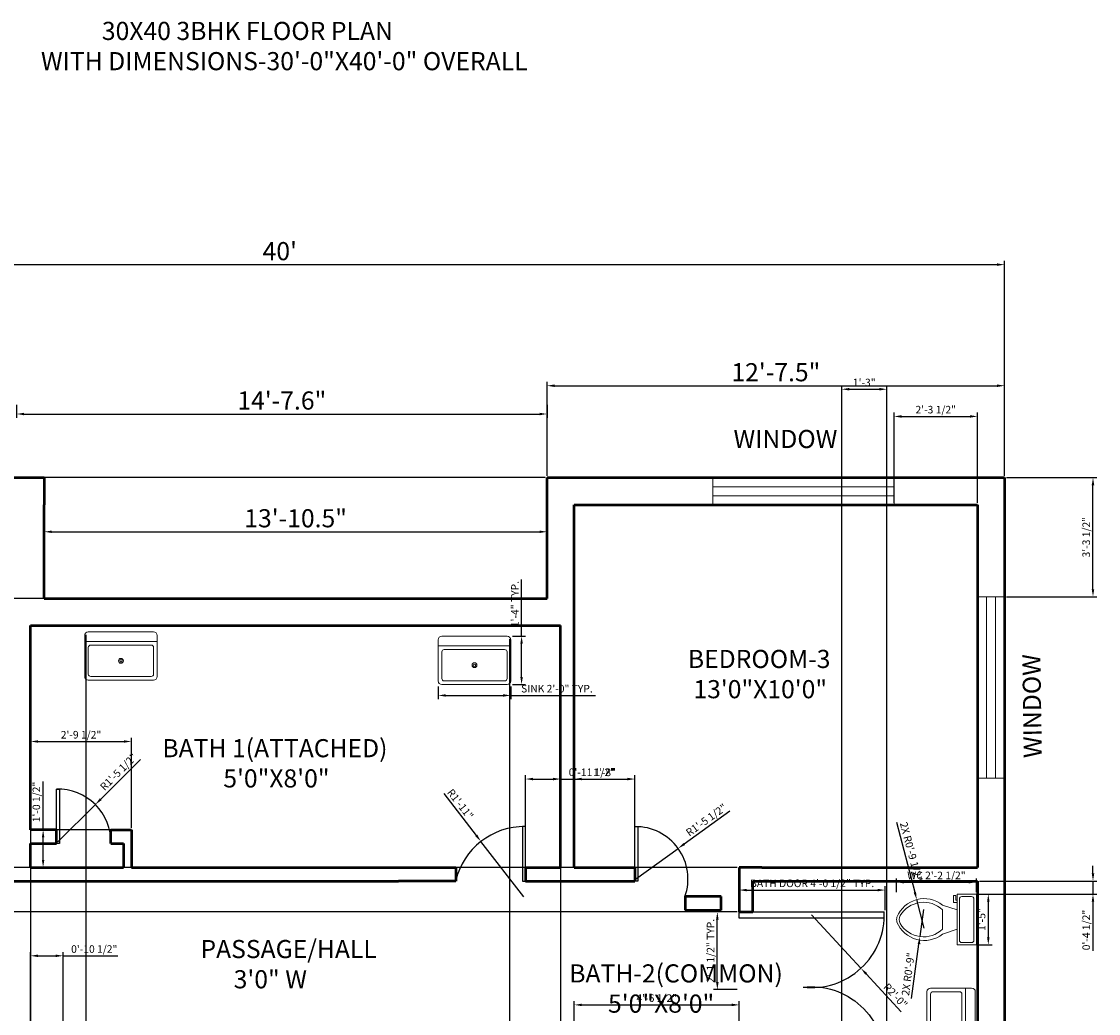
# Model space of a CAD drawing. Units: inches. Extents: x 259417 to 260009, y 246275 to 246915.
# Tile 4 of 4: x 259652 to 260009, y 246587 to 246915. Entities that reach past the tile are written whole.
import ezdxf

# ---------------------------------------------------------------- set-up
doc = ezdxf.new("R2010")
doc.units = ezdxf.units.IN
for name, color, linetype, lineweight in [('A-ANNO-DIMS', 2, 'Continuous', 18), ('A-ANNO-TEXT', 7, 'Continuous', 18), ('A-ANNO-TTLB', 7, 'Continuous', 35), ('A-AREA-IDEN', 7, 'Continuous', 25), ('A-DOOR', 3, 'Continuous', 25), ('A-FLOR-FIXT', 8, 'Continuous', 18), ('A-GLAZ', 4, 'Continuous', 18), ('A-WALL', 7, 'Continuous', 50)]:
    doc.layers.add(name, color=color, linetype=linetype, lineweight=lineweight)
doc.styles.get("Standard").update_dxf_attribs({"font": 'arial.ttf'})
doc.dimstyles.new('ISO-25', dxfattribs={"dimtxt": 2.5, "dimasz": 2.5, "dimexe": 1.25, "dimexo": 0.625, "dimtad": 1, "dimdec": 1, "dimlunit": 3, "dimtxsty": 'Standard', "dimcen": 2.5, "dimadec": 0, "dimazin": 0, "dimtfac": 1, "dimtdec": 1, "dimtmove": 0, "dimatfit": 3, "dimfxl": 1, "dimarcsym": 0})

# ---------------------------------------------------------------- blocks, each defined once
blk = doc.blocks.new('*D8')
at = {"layer": 'A-ANNO-DIMS', "color": 0, "lineweight": -2, "transparency": 16777216}
for p, q in [((259497.59, 246764.47), (259497.59, 246835.57)), ((259500.09, 246834.32), (259975.09, 246834.32)), ((259977.59, 246764.47), (259977.59, 246835.57))]:
    blk.add_line(p, q, dxfattribs=at)
at = {"layer": 'A-ANNO-DIMS', "color": 0, "transparency": 16777216}
for points in [[(259500.09, 246834.74), (259500.09, 246833.91), (259497.59, 246834.32)], [(259975.09, 246834.74), (259975.09, 246833.91), (259977.59, 246834.32)]]:
    blk.add_solid(points, dxfattribs=at)
at = {"layer": 'Defpoints', "color": 0, "transparency": 16777216}
for p in [(259977.59, 246834.32), (259497.59, 246763.84), (259977.59, 246763.84)]:
    blk.add_point(p, dxfattribs=at)
at = {"layer": 'A-ANNO-DIMS', "color": 0, "transparency": 16777216, "insert": (259737.59, 246838.01), "char_height": 6, "attachment_point": 5}
blk.add_mtext("40'", dxfattribs=at)
blk = doc.blocks.new('*D12')
at = {"layer": 'A-ANNO-DIMS', "color": 0, "lineweight": -2, "transparency": 16777216}
for p, q in [((259659.59, 246724.51), (259659.59, 246747.17)), ((259826.09, 246724.51), (259826.09, 246747.17)), ((259662.09, 246745.92), (259823.59, 246745.92))]:
    blk.add_line(p, q, dxfattribs=at)
at = {"layer": 'A-ANNO-DIMS', "color": 0, "transparency": 16777216}
for points in [[(259662.09, 246746.33), (259662.09, 246745.5), (259659.59, 246745.92)], [(259823.59, 246746.33), (259823.59, 246745.5), (259826.09, 246745.92)]]:
    blk.add_solid(points, dxfattribs=at)
at = {"layer": 'Defpoints', "color": 0, "transparency": 16777216}
for p in [(259826.09, 246745.92), (259659.59, 246723.89), (259826.09, 246723.89)]:
    blk.add_point(p, dxfattribs=at)
at = {"layer": 'A-ANNO-DIMS', "color": 0, "transparency": 16777216, "insert": (259742.84, 246749.61), "char_height": 6, "attachment_point": 5}
blk.add_mtext('13\'-10.5"', dxfattribs=at)
blk = doc.blocks.new('*D13')
at = {"layer": 'A-ANNO-DIMS', "color": 0, "lineweight": -2, "transparency": 16777216}
for p, q in [((259826.09, 246764.47), (259826.09, 246795.5)), ((259828.59, 246794.25), (259975.09, 246794.25)), ((259977.59, 246764.47), (259977.59, 246795.5))]:
    blk.add_line(p, q, dxfattribs=at)
at = {"layer": 'A-ANNO-DIMS', "color": 0, "transparency": 16777216}
for points in [[(259828.59, 246794.67), (259828.59, 246793.84), (259826.09, 246794.25)], [(259975.09, 246794.67), (259975.09, 246793.84), (259977.59, 246794.25)]]:
    blk.add_solid(points, dxfattribs=at)
at = {"layer": 'Defpoints', "color": 0, "transparency": 16777216}
for p in [(259977.59, 246794.25), (259826.09, 246763.84), (259977.59, 246763.84)]:
    blk.add_point(p, dxfattribs=at)
at = {"layer": 'A-ANNO-DIMS', "color": 0, "transparency": 16777216, "insert": (259901.84, 246797.94), "char_height": 6, "attachment_point": 5}
blk.add_mtext('12\'-7.5"', dxfattribs=at)
blk = doc.blocks.new('*D14')
at = {"layer": 'A-ANNO-DIMS', "color": 0, "lineweight": -2, "transparency": 16777216}
for p, q in [((259650.46, 246787.95), (259650.46, 246783.64)), ((259826.09, 246787.95), (259826.09, 246783.64)), ((259652.96, 246784.89), (259823.59, 246784.89))]:
    blk.add_line(p, q, dxfattribs=at)
at = {"layer": 'A-ANNO-DIMS', "color": 0, "transparency": 16777216}
for points in [[(259652.96, 246785.31), (259652.96, 246784.47), (259650.46, 246784.89)], [(259823.59, 246785.31), (259823.59, 246784.47), (259826.09, 246784.89)]]:
    blk.add_solid(points, dxfattribs=at)
at = {"layer": 'Defpoints', "color": 0, "transparency": 16777216}
for p in [(259650.46, 246788.57), (259826.09, 246788.57), (259826.09, 246784.89)]:
    blk.add_point(p, dxfattribs=at)
at = {"layer": 'A-ANNO-DIMS', "color": 0, "transparency": 16777216, "insert": (259738.27, 246788.58), "char_height": 6, "attachment_point": 5}
blk.add_mtext('14\'-7.6"', dxfattribs=at)
blk = doc.blocks.new('Toilet - top')
for p, q in [((9.5, -6), (9.5, -2)), ((-10, -8.5), (-8, -8.5)), ((-10, -9.5), (-10, -8.5)), ((-8, -8.5), (-8, -8)), ((-7, -8), (-7, -9.5)), ((-4, -8), (-6, -14)), ((4, -8), (6, -14)), ((-7, -9.5), (-10, -9.5)), ((4, -14), (-4, -14))]:
    blk.add_line(p, q)
blk.add_lwpolyline([(10.5, -8), (10.5, 0), (-10.5, 0), (-10.5, -8)], close=True)
for points in [[(-9.5, -2), (-9.5, -6)], [(8.5, -1), (-8.5, -1)], [(-8.5, -7), (8.5, -7)]]:
    blk.add_lwpolyline(points)
for centre, radius, start, end in [((-8.62, -1.88), 0.884, 81.8699, 188.1301), ((8.62, -1.88), 0.884, 351.8699, 98.1301), ((-8.62, -6.12), 0.884, 171.8699, 278.1301), ((8.62, -6.12), 0.884, 261.8699, 8.1301), ((3.52, -21.58), 12.17, 141.4691, 247.9714), ((4.2, -21.82), 11.33, 136.3677, 238.9468), ((-3.52, -21.58), 12.17, 292.0284, 38.5307), ((-4.2, -21.82), 11.33, 301.053, 43.6321), ((0, -27.88), 4, 245.7318, 294.2682), ((0, -29), 4, 254.8605, 285.1395)]:
    blk.add_arc(centre, radius, start, end)
blk = doc.blocks.new('Sink-single - 30 in top')
blk.add_line((-15, -3.999996), (15, -3.999996))
for points in [[(-13.5, 0), (13.5, 0)], [(-15, -18.499996), (-15, -1.5)], [(15, -1.5), (15, -18.499996)], [(-13.5, -17.499996), (-13.5, -6.499996)], [(-12.5, -5.499996), (12.5, -5.499996)], [(13.5, -6.499996), (13.5, -17.499996)], [(13.5, -19.999996), (-13.5, -19.999996)], [(12.5, -18.499996), (-12.5, -18.499996)]]:
    blk.add_lwpolyline(points)
for radius in [1, 0.5]:
    blk.add_circle((0, -11.999996), radius)
for centre, radius, start, end in [((-13.5, -1.5), 1.5, 90, 180), ((13.5, -1.5), 1.5, 0, 90), ((-12.5, -6.499996), 1, 90, 180), ((12.5, -6.499996), 1, 0, 90), ((-12.5, -17.499996), 1, 180, 270), ((12.5, -17.499996), 1, 270, 0), ((-13.5, -18.499996), 1.5, 180, 270), ((13.5, -18.499996), 1.5, 270, 0)]:
    blk.add_arc(centre, radius, start, end)
blk = doc.blocks.new('WIN-60x9')
for p, q in [((0, 9), (0, 0)), ((60, 9), (60, 0)), ((60, 6), (0, 6)), ((60, 3), (0, 3))]:
    blk.add_line(p, q)
blk = doc.blocks.new('DOOR-BATH-PAIRED-LEAF')
for p, q in [((0, 0), (48, 0)), ((0, -2), (0, 0)), ((48, -2), (0, -2)), ((48, -2), (48, 0))]:
    blk.add_line(p, q)
blk.add_arc((23.97, -1), 24.05, 263.254, 2.3829)
blk = doc.blocks.new('*D26')
at = {"layer": 'A-ANNO-DIMS', "color": 0, "lineweight": -2, "transparency": 16777216}
for p, q in [((259790.05, 246694.73), (259790.05, 246690.51)), ((259814.05, 246694.73), (259814.05, 246690.51)), ((259792.55, 246691.76), (259811.55, 246691.76)), ((259814.05, 246691.76), (259842.15, 246691.76))]:
    blk.add_line(p, q, dxfattribs=at)
at = {"layer": 'A-ANNO-DIMS', "color": 0, "transparency": 16777216}
for points in [[(259792.55, 246692.17), (259792.55, 246691.34), (259790.05, 246691.76)], [(259811.55, 246692.17), (259811.55, 246691.34), (259814.05, 246691.76)]]:
    blk.add_solid(points, dxfattribs=at)
at = {"layer": 'Defpoints', "color": 0, "transparency": 16777216}
for p in [(259790.05, 246695.36), (259814.05, 246695.36), (259814.05, 246691.76)]:
    blk.add_point(p, dxfattribs=at)
at = {"layer": 'A-ANNO-DIMS', "color": 0, "transparency": 16777216, "insert": (259829.35, 246693.67), "char_height": 2.5, "attachment_point": 5}
blk.add_mtext('SINK 2\'-0" TYP.', dxfattribs=at)
blk = doc.blocks.new('*D27')
at = {"layer": 'A-ANNO-DIMS', "color": 0, "lineweight": -2, "transparency": 16777216}
for p, q in [((259817.65, 246711.36), (259817.65, 246730.11)), ((259814.67, 246711.36), (259818.9, 246711.36)), ((259817.65, 246697.86), (259817.65, 246708.86)), ((259814.67, 246695.36), (259818.9, 246695.36))]:
    blk.add_line(p, q, dxfattribs=at)
at = {"layer": 'A-ANNO-DIMS', "color": 0, "transparency": 16777216}
for points in [[(259817.23, 246708.86), (259818.07, 246708.86), (259817.65, 246711.36)], [(259817.23, 246697.86), (259818.07, 246697.86), (259817.65, 246695.36)]]:
    blk.add_solid(points, dxfattribs=at)
at = {"layer": 'Defpoints', "color": 0, "transparency": 16777216}
for p in [(259814.05, 246711.36), (259817.65, 246711.36), (259814.05, 246695.36)]:
    blk.add_point(p, dxfattribs=at)
at = {"layer": 'A-ANNO-DIMS', "color": 0, "transparency": 16777216, "insert": (259815.77, 246721.98), "char_height": 2.5, "attachment_point": 5, "rotation": 90}
blk.add_mtext('1\'-4" TYP.', dxfattribs=at)
blk = doc.blocks.new('*D28')
at = {"layer": 'A-ANNO-DIMS', "color": 0, "lineweight": -2, "transparency": 16777216}
for p, q in [((259889.71, 246620.72), (259889.71, 246628.59)), ((259892.21, 246627.34), (259935.5, 246627.34)), ((259938, 246620.72), (259938, 246628.59))]:
    blk.add_line(p, q, dxfattribs=at)
at = {"layer": 'A-ANNO-DIMS', "color": 0, "transparency": 16777216}
for points in [[(259892.21, 246627.76), (259892.21, 246626.93), (259889.71, 246627.34)], [(259935.5, 246627.76), (259935.5, 246626.93), (259938, 246627.34)]]:
    blk.add_solid(points, dxfattribs=at)
at = {"layer": 'Defpoints', "color": 0, "transparency": 16777216}
for p in [(259938, 246627.34), (259889.71, 246620.1), (259938, 246620.1)]:
    blk.add_point(p, dxfattribs=at)
at = {"layer": 'A-ANNO-DIMS', "color": 0, "transparency": 16777216, "insert": (259913.85, 246629.26), "char_height": 2.5, "attachment_point": 5}
blk.add_mtext('BATH DOOR 4\'-0 1/2" TYP.', dxfattribs=at)
blk = doc.blocks.new('*D29')
at = {"layer": 'A-ANNO-DIMS', "color": 0, "lineweight": -2, "transparency": 16777216}
for p, q in [((259889.08, 246620.1), (259881.21, 246620.1)), ((259882.46, 246596.89), (259882.46, 246617.6)), ((259889.08, 246594.39), (259881.21, 246594.39))]:
    blk.add_line(p, q, dxfattribs=at)
at = {"layer": 'A-ANNO-DIMS', "color": 0, "transparency": 16777216}
for points in [[(259882.05, 246617.6), (259882.88, 246617.6), (259882.46, 246620.1)], [(259882.05, 246596.89), (259882.88, 246596.89), (259882.46, 246594.39)]]:
    blk.add_solid(points, dxfattribs=at)
at = {"layer": 'Defpoints', "color": 0, "transparency": 16777216}
for p in [(259882.46, 246620.1), (259889.71, 246620.1), (259889.71, 246594.39)]:
    blk.add_point(p, dxfattribs=at)
at = {"layer": 'A-ANNO-DIMS', "color": 0, "transparency": 16777216, "insert": (259880.54, 246607.24), "char_height": 2.5, "attachment_point": 5, "rotation": 90}
blk.add_mtext('2\'-1 1/2" TYP.', dxfattribs=at)
blk = doc.blocks.new('*D32')
at = {"layer": 'A-ANNO-DIMS', "color": 0, "lineweight": -2, "transparency": 16777216}
for p, q in [((259941.78, 246626.62), (259941.78, 246631.21)), ((259944.28, 246629.96), (259965.72, 246629.96)), ((259968.22, 246626.62), (259968.22, 246631.21))]:
    blk.add_line(p, q, dxfattribs=at)
at = {"layer": 'A-ANNO-DIMS', "color": 0, "transparency": 16777216}
for points in [[(259944.28, 246630.38), (259944.28, 246629.54), (259941.78, 246629.96)], [(259965.72, 246630.38), (259965.72, 246629.54), (259968.22, 246629.96)]]:
    blk.add_solid(points, dxfattribs=at)
at = {"layer": 'Defpoints', "color": 0, "transparency": 16777216}
for p in [(259968.22, 246629.96), (259941.78, 246625.99), (259968.22, 246625.99)]:
    blk.add_point(p, dxfattribs=at)
at = {"layer": 'A-ANNO-DIMS', "color": 0, "transparency": 16777216, "insert": (259955, 246631.88), "char_height": 2.5, "attachment_point": 5}
blk.add_mtext('WC 2\'-2 1/2"', dxfattribs=at)
blk = doc.blocks.new('*D33')
at = {"layer": 'A-ANNO-DIMS', "color": 0, "lineweight": -2, "transparency": 16777216}
for p, q in [((259968.84, 246625.99), (259973.43, 246625.99)), ((259972.18, 246623.49), (259972.18, 246611.69)), ((259968.84, 246609.19), (259973.43, 246609.19))]:
    blk.add_line(p, q, dxfattribs=at)
at = {"layer": 'A-ANNO-DIMS', "color": 0, "transparency": 16777216}
for points in [[(259971.77, 246623.49), (259972.6, 246623.49), (259972.18, 246625.99)], [(259971.77, 246611.69), (259972.6, 246611.69), (259972.18, 246609.19)]]:
    blk.add_solid(points, dxfattribs=at)
at = {"layer": 'Defpoints', "color": 0, "transparency": 16777216}
for p in [(259968.22, 246625.99), (259968.22, 246609.19), (259972.18, 246609.19)]:
    blk.add_point(p, dxfattribs=at)
at = {"layer": 'A-ANNO-DIMS', "color": 0, "transparency": 16777216, "insert": (259970.28, 246617.59), "char_height": 2.5, "attachment_point": 5, "rotation": 90}
blk.add_mtext('1\'-5"', dxfattribs=at)
blk = doc.blocks.new('*D35')
at = {"layer": 'A-ANNO-DIMS', "color": 0, "lineweight": -2, "transparency": 16777216}
for p, q in [((259940.97, 246755.47), (259940.97, 246785.34)), ((259943.47, 246784.09), (259966.09, 246784.09)), ((259968.59, 246755.47), (259968.59, 246785.34))]:
    blk.add_line(p, q, dxfattribs=at)
at = {"layer": 'A-ANNO-DIMS', "color": 0, "transparency": 16777216}
for points in [[(259943.47, 246784.51), (259943.47, 246783.67), (259940.97, 246784.09)], [(259966.09, 246784.51), (259966.09, 246783.67), (259968.59, 246784.09)]]:
    blk.add_solid(points, dxfattribs=at)
at = {"layer": 'Defpoints', "color": 0, "transparency": 16777216}
for p in [(259968.59, 246784.09), (259940.97, 246754.84), (259968.59, 246754.84)]:
    blk.add_point(p, dxfattribs=at)
at = {"layer": 'A-ANNO-DIMS', "color": 0, "transparency": 16777216, "insert": (259954.78, 246786.01), "char_height": 2.5, "attachment_point": 5}
blk.add_mtext('2\'-3 1/2"', dxfattribs=at)
blk = doc.blocks.new('*D36')
at = {"layer": 'A-ANNO-DIMS', "color": 0, "lineweight": -2, "transparency": 16777216}
for p, q in [((259978.22, 246763.84), (260008.09, 246763.84)), ((260006.84, 246726.92), (260006.84, 246761.34)), ((259978.22, 246724.42), (260008.09, 246724.42))]:
    blk.add_line(p, q, dxfattribs=at)
at = {"layer": 'A-ANNO-DIMS', "color": 0, "transparency": 16777216}
for points in [[(260006.42, 246761.34), (260007.26, 246761.34), (260006.84, 246763.84)], [(260006.42, 246726.92), (260007.26, 246726.92), (260006.84, 246724.42)]]:
    blk.add_solid(points, dxfattribs=at)
at = {"layer": 'Defpoints', "color": 0, "transparency": 16777216}
for p in [(259977.59, 246763.84), (260006.84, 246763.84), (259977.59, 246724.42)]:
    blk.add_point(p, dxfattribs=at)
at = {"layer": 'A-ANNO-DIMS', "color": 0, "transparency": 16777216, "insert": (260004.92, 246744.13), "char_height": 2.5, "attachment_point": 5, "rotation": 90}
blk.add_mtext('3\'-3 1/2"', dxfattribs=at)
blk = doc.blocks.new('*D42')
at = {"layer": 'A-ANNO-DIMS', "color": 0, "lineweight": -2, "transparency": 16777216}
for p, q in [((259825.47, 246763.84), (259429.27, 246763.84)), ((259430.52, 246761.34), (259430.52, 246726.39)), ((259825.47, 246723.89), (259429.27, 246723.89))]:
    blk.add_line(p, q, dxfattribs=at)
at = {"layer": 'A-ANNO-DIMS', "color": 0, "transparency": 16777216}
for points in [[(259430.11, 246761.34), (259430.94, 246761.34), (259430.52, 246763.84)], [(259430.11, 246726.39), (259430.94, 246726.39), (259430.52, 246723.89)]]:
    blk.add_solid(points, dxfattribs=at)
at = {"layer": 'Defpoints', "color": 0, "transparency": 16777216}
for p in [(259826.09, 246763.84), (259430.52, 246723.89), (259826.09, 246723.89)]:
    blk.add_point(p, dxfattribs=at)
at = {"layer": 'A-ANNO-DIMS', "color": 0, "transparency": 16777216, "insert": (259428.62, 246743.87), "char_height": 2.5, "attachment_point": 5, "rotation": 90}
blk.add_mtext('3\'-4"', dxfattribs=at)
blk = doc.blocks.new('*D49')
at = {"layer": 'A-ANNO-DIMS', "color": 0, "lineweight": -2, "transparency": 16777216}
for p, q in [((259835.09, 246560.72), (259835.09, 246590.6)), ((259889.71, 246560.72), (259889.71, 246590.6)), ((259837.59, 246589.35), (259887.21, 246589.35))]:
    blk.add_line(p, q, dxfattribs=at)
at = {"layer": 'A-ANNO-DIMS', "color": 0, "transparency": 16777216}
for points in [[(259837.59, 246589.77), (259837.59, 246588.93), (259835.09, 246589.35)], [(259887.21, 246589.77), (259887.21, 246588.93), (259889.71, 246589.35)]]:
    blk.add_solid(points, dxfattribs=at)
at = {"layer": 'Defpoints', "color": 0, "transparency": 16777216}
for p in [(259889.71, 246589.35), (259835.09, 246560.1), (259889.71, 246560.1)]:
    blk.add_point(p, dxfattribs=at)
at = {"layer": 'A-ANNO-DIMS', "color": 0, "transparency": 16777216, "insert": (259862.4, 246591.27), "char_height": 2.5, "attachment_point": 5}
blk.add_mtext('4\'-6 1/2"', dxfattribs=at)
blk = doc.blocks.new('*D51')
at = {"layer": 'A-ANNO-DIMS', "color": 0, "lineweight": -2, "transparency": 16777216}
for p, q in [((259818.94, 246635.47), (259818.94, 246665.34)), ((259830.59, 246635.47), (259830.59, 246665.34)), ((259821.44, 246664.09), (259828.09, 246664.09)), ((259830.59, 246664.09), (259848.75, 246664.09))]:
    blk.add_line(p, q, dxfattribs=at)
at = {"layer": 'A-ANNO-DIMS', "color": 0, "transparency": 16777216}
for points in [[(259821.44, 246664.51), (259821.44, 246663.67), (259818.94, 246664.09)], [(259828.09, 246664.51), (259828.09, 246663.67), (259830.59, 246664.09)]]:
    blk.add_solid(points, dxfattribs=at)
at = {"layer": 'Defpoints', "color": 0, "transparency": 16777216}
for p in [(259830.59, 246664.09), (259818.94, 246634.84), (259830.59, 246634.84)]:
    blk.add_point(p, dxfattribs=at)
at = {"layer": 'A-ANNO-DIMS', "color": 0, "transparency": 16777216, "insert": (259840.92, 246666.01), "char_height": 2.5, "attachment_point": 5}
blk.add_mtext('0\'-11 1/2"', dxfattribs=at)
blk = doc.blocks.new('*D52')
at = {"layer": 'A-ANNO-DIMS', "color": 0, "lineweight": -2, "transparency": 16777216}
for p, q in [((259835.09, 246635.47), (259835.09, 246665.34)), ((259855.17, 246635.47), (259855.17, 246665.34)), ((259837.59, 246664.09), (259852.67, 246664.09))]:
    blk.add_line(p, q, dxfattribs=at)
at = {"layer": 'A-ANNO-DIMS', "color": 0, "transparency": 16777216}
for points in [[(259837.59, 246664.51), (259837.59, 246663.67), (259835.09, 246664.09)], [(259852.67, 246664.51), (259852.67, 246663.67), (259855.17, 246664.09)]]:
    blk.add_solid(points, dxfattribs=at)
at = {"layer": 'Defpoints', "color": 0, "transparency": 16777216}
for p in [(259855.17, 246664.09), (259835.09, 246634.84), (259855.17, 246634.84)]:
    blk.add_point(p, dxfattribs=at)
at = {"layer": 'A-ANNO-DIMS', "color": 0, "transparency": 16777216, "insert": (259845.13, 246665.99), "char_height": 2.5, "attachment_point": 5}
blk.add_mtext('1\'-8"', dxfattribs=at)
blk = doc.blocks.new('*D53')
at = {"layer": 'A-ANNO-DIMS', "color": 0, "lineweight": -2, "transparency": 16777216}
for p, q in [((259655.09, 246576.97), (259655.09, 246606.84)), ((259657.59, 246605.59), (259663.34, 246605.59)), ((259665.84, 246576.97), (259665.84, 246606.84)), ((259665.84, 246605.59), (259684, 246605.59))]:
    blk.add_line(p, q, dxfattribs=at)
at = {"layer": 'A-ANNO-DIMS', "color": 0, "transparency": 16777216}
for points in [[(259657.59, 246606.01), (259657.59, 246605.17), (259655.09, 246605.59)], [(259663.34, 246606.01), (259663.34, 246605.17), (259665.84, 246605.59)]]:
    blk.add_solid(points, dxfattribs=at)
at = {"layer": 'Defpoints', "color": 0, "transparency": 16777216}
for p in [(259665.84, 246605.59), (259655.09, 246576.34), (259665.84, 246576.34)]:
    blk.add_point(p, dxfattribs=at)
at = {"layer": 'A-ANNO-DIMS', "color": 0, "transparency": 16777216, "insert": (259676.17, 246607.51), "char_height": 2.5, "attachment_point": 5}
blk.add_mtext('0\'-10 1/2"', dxfattribs=at)
blk = doc.blocks.new('*D55')
at = {"layer": 'A-ANNO-DIMS', "color": 0, "lineweight": -2, "transparency": 16777216}
for p, q in [((259889.08, 246634.84), (259429.27, 246634.84)), ((259430.52, 246622.6), (259430.52, 246632.34)), ((259889.08, 246620.1), (259429.27, 246620.1))]:
    blk.add_line(p, q, dxfattribs=at)
at = {"layer": 'A-ANNO-DIMS', "color": 0, "transparency": 16777216}
for points in [[(259430.11, 246632.34), (259430.94, 246632.34), (259430.52, 246634.84)], [(259430.11, 246622.6), (259430.94, 246622.6), (259430.52, 246620.1)]]:
    blk.add_solid(points, dxfattribs=at)
at = {"layer": 'Defpoints', "color": 0, "transparency": 16777216}
for p in [(259430.52, 246634.84), (259889.71, 246634.84), (259889.71, 246620.1)]:
    blk.add_point(p, dxfattribs=at)
at = {"layer": 'A-ANNO-DIMS', "color": 0, "transparency": 16777216, "insert": (259428.61, 246627.47), "char_height": 2.5, "attachment_point": 5, "rotation": 90}
blk.add_mtext('1\'-2 1/2"', dxfattribs=at)
blk = doc.blocks.new('*D57')
at = {"layer": 'A-ANNO-DIMS', "color": 0, "lineweight": -2, "transparency": 16777216}
for p, q in [((260006.84, 246632.84), (260006.84, 246635.34)), ((259969.22, 246630.34), (260008.09, 246630.34)), ((260006.84, 246630.34), (260006.84, 246625.99)), ((259968.84, 246625.99), (260008.09, 246625.99)), ((260006.84, 246623.49), (260006.84, 246607.27))]:
    blk.add_line(p, q, dxfattribs=at)
at = {"layer": 'A-ANNO-DIMS', "color": 0, "transparency": 16777216}
for points in [[(260006.42, 246632.84), (260007.26, 246632.84), (260006.84, 246630.34)], [(260006.42, 246623.49), (260007.26, 246623.49), (260006.84, 246625.99)]]:
    blk.add_solid(points, dxfattribs=at)
at = {"layer": 'Defpoints', "color": 0, "transparency": 16777216}
for p in [(259968.59, 246630.34), (259968.22, 246625.99), (260006.84, 246625.99)]:
    blk.add_point(p, dxfattribs=at)
at = {"layer": 'A-ANNO-DIMS', "color": 0, "transparency": 16777216, "insert": (260004.92, 246614.13), "char_height": 2.5, "attachment_point": 5, "rotation": 90}
blk.add_mtext('0\'-4 1/2"', dxfattribs=at)
blk = doc.blocks.new('*D59')
at = {"layer": 'A-ANNO-DIMS', "color": 0, "lineweight": -2, "transparency": 16777216}
for p, q in [((259923.64, 246415.68), (259923.64, 246794.34)), ((259938.59, 246413.47), (259938.59, 246794.34)), ((259926.14, 246793.09), (259936.09, 246793.09))]:
    blk.add_line(p, q, dxfattribs=at)
at = {"layer": 'A-ANNO-DIMS', "color": 0, "transparency": 16777216}
for points in [[(259926.14, 246793.51), (259926.14, 246792.67), (259923.64, 246793.09)], [(259936.09, 246793.51), (259936.09, 246792.67), (259938.59, 246793.09)]]:
    blk.add_solid(points, dxfattribs=at)
at = {"layer": 'Defpoints', "color": 0, "transparency": 16777216}
for p in [(259938.59, 246793.09), (259923.64, 246415.05), (259938.59, 246412.84)]:
    blk.add_point(p, dxfattribs=at)
at = {"layer": 'A-ANNO-DIMS', "color": 0, "transparency": 16777216, "insert": (259931.11, 246794.99), "char_height": 2.5, "attachment_point": 5}
blk.add_mtext('1\'-3"', dxfattribs=at)
blk = doc.blocks.new('*D60')
at = {"layer": 'A-ANNO-DIMS', "color": 0, "lineweight": -2, "transparency": 16777216}
for p, q in [((259655.09, 246647.89), (259655.09, 246677.76)), ((259657.59, 246676.51), (259685.99, 246676.51)), ((259688.49, 246647.89), (259688.49, 246677.76))]:
    blk.add_line(p, q, dxfattribs=at)
at = {"layer": 'A-ANNO-DIMS', "color": 0, "transparency": 16777216}
for points in [[(259657.59, 246676.93), (259657.59, 246676.1), (259655.09, 246676.51)], [(259685.99, 246676.93), (259685.99, 246676.1), (259688.49, 246676.51)]]:
    blk.add_solid(points, dxfattribs=at)
at = {"layer": 'Defpoints', "color": 0, "transparency": 16777216}
for p in [(259688.49, 246676.51), (259655.09, 246647.26), (259688.49, 246647.26)]:
    blk.add_point(p, dxfattribs=at)
at = {"layer": 'A-ANNO-DIMS', "color": 0, "transparency": 16777216, "insert": (259671.79, 246678.43), "char_height": 2.5, "attachment_point": 5}
blk.add_mtext('2\'-9 1/2"', dxfattribs=at)
blk = doc.blocks.new('*D61')
at = {"layer": 'A-ANNO-DIMS', "color": 0, "lineweight": -2, "transparency": 16777216}
for p, q in [((259659.24, 246647.26), (259659.24, 246663.25)), ((259687.86, 246647.26), (259657.99, 246647.26)), ((259659.24, 246637.34), (259659.24, 246644.76)), ((259687.86, 246634.84), (259657.99, 246634.84))]:
    blk.add_line(p, q, dxfattribs=at)
at = {"layer": 'A-ANNO-DIMS', "color": 0, "transparency": 16777216}
for points in [[(259658.82, 246644.76), (259659.65, 246644.76), (259659.24, 246647.26)], [(259658.82, 246637.34), (259659.65, 246637.34), (259659.24, 246634.84)]]:
    blk.add_solid(points, dxfattribs=at)
at = {"layer": 'Defpoints', "color": 0, "transparency": 16777216}
for p in [(259659.24, 246647.26), (259688.49, 246647.26), (259688.49, 246634.84)]:
    blk.add_point(p, dxfattribs=at)
at = {"layer": 'A-ANNO-DIMS', "color": 0, "transparency": 16777216, "insert": (259657.32, 246656.5), "char_height": 2.5, "attachment_point": 5, "rotation": 90}
blk.add_mtext('1\'-0 1/2"', dxfattribs=at)
blk = doc.blocks.new('*D62')
at = {"layer": 'A-ANNO-DIMS', "color": 0, "lineweight": -2, "transparency": 16777216}
for p, q in [((259655.09, 246714.26), (259655.09, 246340.98)), ((259673.35, 246711.84), (259673.35, 246340.98)), ((259657.59, 246342.23), (259670.85, 246342.23))]:
    blk.add_line(p, q, dxfattribs=at)
at = {"layer": 'A-ANNO-DIMS', "color": 0, "transparency": 16777216}
for points in [[(259657.59, 246342.64), (259657.59, 246341.81), (259655.09, 246342.23)], [(259670.85, 246342.64), (259670.85, 246341.81), (259673.35, 246342.23)]]:
    blk.add_solid(points, dxfattribs=at)
at = {"layer": 'Defpoints', "color": 0, "transparency": 16777216}
for p in [(259655.09, 246714.89), (259673.35, 246712.46), (259673.35, 246342.23)]:
    blk.add_point(p, dxfattribs=at)
at = {"layer": 'A-ANNO-DIMS', "color": 0, "transparency": 16777216, "insert": (259664.22, 246344.15), "char_height": 2.5, "attachment_point": 5}
blk.add_mtext('1\'-6 1/2"', dxfattribs=at)
blk = doc.blocks.new('*D63')
at = {"layer": 'A-ANNO-DIMS', "color": 0, "lineweight": -2, "transparency": 16777216}
for p, q in [((259830.59, 246714.26), (259830.59, 246340.98)), ((259813.7, 246710.38), (259813.7, 246340.98)), ((259816.2, 246342.23), (259828.09, 246342.23))]:
    blk.add_line(p, q, dxfattribs=at)
at = {"layer": 'A-ANNO-DIMS', "color": 0, "transparency": 16777216}
for points in [[(259816.2, 246342.64), (259816.2, 246341.81), (259813.7, 246342.23)], [(259828.09, 246342.64), (259828.09, 246341.81), (259830.59, 246342.23)]]:
    blk.add_solid(points, dxfattribs=at)
at = {"layer": 'Defpoints', "color": 0, "transparency": 16777216}
for p in [(259830.59, 246714.89), (259813.7, 246711.01), (259830.59, 246342.23)]:
    blk.add_point(p, dxfattribs=at)
at = {"layer": 'A-ANNO-DIMS', "color": 0, "transparency": 16777216, "insert": (259822.14, 246344.13), "char_height": 2.5, "attachment_point": 5}
blk.add_mtext('1\'-5"', dxfattribs=at)
blk = doc.blocks.new('*D68')
at = {"layer": 'A-ANNO-DIMS', "color": 0, "lineweight": -2, "transparency": 16777216}
for p, q in [((259913.68, 246619.1), (259930.02, 246601.46)), ((259943.33, 246587.1), (259931.72, 246599.62))]:
    blk.add_line(p, q, dxfattribs=at)
at = {"layer": 'A-ANNO-DIMS', "color": 0, "transparency": 16777216}
blk.add_solid([(259932.03, 246599.91), (259931.42, 246599.34), (259930.02, 246601.46)], dxfattribs=at)
at = {"layer": 'Defpoints', "color": 0, "transparency": 16777216}
for p in [(259913.68, 246619.1), (259930.02, 246601.46)]:
    blk.add_point(p, dxfattribs=at)
at = {"layer": 'A-ANNO-DIMS', "color": 0, "transparency": 16777216, "insert": (259941.23, 246592.17), "char_height": 2.5, "attachment_point": 5, "rotation": 312.8183}
blk.add_mtext('R2\'-0"', dxfattribs=at)
blk = doc.blocks.new('*D69')
at = {"layer": 'A-ANNO-DIMS', "color": 0, "lineweight": -2, "transparency": 16777216}
for p, q in [((259791.87, 246659.26), (259802.65, 246645.42)), ((259818.44, 246625.14), (259804.19, 246643.45))]:
    blk.add_line(p, q, dxfattribs=at)
at = {"layer": 'A-ANNO-DIMS', "color": 0, "transparency": 16777216}
blk.add_solid([(259802.98, 246645.68), (259802.32, 246645.17), (259804.19, 246643.45)], dxfattribs=at)
at = {"layer": 'Defpoints', "color": 0, "transparency": 16777216}
for p in [(259804.19, 246643.45), (259818.44, 246625.14)]:
    blk.add_point(p, dxfattribs=at)
at = {"layer": 'A-ANNO-DIMS', "color": 0, "transparency": 16777216, "insert": (259797.12, 246655.59), "char_height": 2.5, "attachment_point": 5, "rotation": 307.9112}
blk.add_mtext('R1\'-11"', dxfattribs=at)
blk = doc.blocks.new('*D70')
at = {"layer": 'A-ANNO-DIMS', "color": 0, "lineweight": -2, "transparency": 16777216}
for p, q in [((259691.46, 246670.57), (259678.3, 246657.41)), ((259664.15, 246643.26), (259676.53, 246655.64))]:
    blk.add_line(p, q, dxfattribs=at)
at = {"layer": 'A-ANNO-DIMS', "color": 0, "transparency": 16777216}
blk.add_solid([(259678, 246657.7), (259678.59, 246657.11), (259676.53, 246655.64)], dxfattribs=at)
at = {"layer": 'Defpoints', "color": 0, "transparency": 16777216}
for p in [(259676.53, 246655.64), (259664.15, 246643.26)]:
    blk.add_point(p, dxfattribs=at)
at = {"layer": 'A-ANNO-DIMS', "color": 0, "transparency": 16777216, "insert": (259684.41, 246666.23), "char_height": 2.5, "attachment_point": 5, "rotation": 44.9986}
blk.add_mtext('R1\'-5 1/2"', dxfattribs=at)
blk = doc.blocks.new('*D71')
at = {"layer": 'A-ANNO-DIMS', "color": 0, "lineweight": -2, "transparency": 16777216}
for p, q in [((259886.65, 246653.43), (259871.53, 246642.58)), ((259855.42, 246631.01), (259869.5, 246641.12))]:
    blk.add_line(p, q, dxfattribs=at)
at = {"layer": 'A-ANNO-DIMS', "color": 0, "transparency": 16777216}
blk.add_solid([(259871.29, 246642.91), (259871.77, 246642.24), (259869.5, 246641.12)], dxfattribs=at)
at = {"layer": 'Defpoints', "color": 0, "transparency": 16777216}
for p in [(259869.5, 246641.12), (259855.42, 246631.01)]:
    blk.add_point(p, dxfattribs=at)
at = {"layer": 'A-ANNO-DIMS', "color": 0, "transparency": 16777216, "insert": (259878.99, 246650.29), "char_height": 2.5, "attachment_point": 5, "rotation": 35.6707}
blk.add_mtext('R1\'-5 1/2"', dxfattribs=at)
blk = doc.blocks.new('*D72')
at = {"layer": 'A-ANNO-DIMS', "color": 0, "lineweight": -2, "transparency": 16777216}
for p, q in [((259941.74, 246649.85), (259947.84, 246626.61)), ((259950.95, 246614.78), (259948.48, 246624.19))]:
    blk.add_line(p, q, dxfattribs=at)
at = {"layer": 'A-ANNO-DIMS', "color": 0, "transparency": 16777216}
blk.add_solid([(259948.25, 246626.72), (259947.44, 246626.51), (259948.48, 246624.19)], dxfattribs=at)
at = {"layer": 'Defpoints', "color": 0, "transparency": 16777216}
for p in [(259948.48, 246624.19), (259950.95, 246614.78)]:
    blk.add_point(p, dxfattribs=at)
at = {"layer": 'A-ANNO-DIMS', "color": 0, "transparency": 16777216, "insert": (259946.33, 246639.93), "char_height": 2.5, "attachment_point": 5, "rotation": 284.7174}
blk.add_mtext('2X R0\'-9 1/2"', dxfattribs=at)
blk = doc.blocks.new('*D73')
at = {"layer": 'A-ANNO-DIMS', "color": 0, "lineweight": -2, "transparency": 16777216}
for p, q in [((259950.76, 246620.95), (259949.56, 246611.97)), ((259946.8, 246591.45), (259949.22, 246609.49))]:
    blk.add_line(p, q, dxfattribs=at)
at = {"layer": 'A-ANNO-DIMS', "color": 0, "transparency": 16777216}
blk.add_solid([(259948.81, 246609.55), (259949.63, 246609.44), (259949.56, 246611.97)], dxfattribs=at)
at = {"layer": 'Defpoints', "color": 0, "transparency": 16777216}
for p in [(259950.76, 246620.95), (259949.56, 246611.97)]:
    blk.add_point(p, dxfattribs=at)
at = {"layer": 'A-ANNO-DIMS', "color": 0, "transparency": 16777216, "insert": (259945.96, 246599.49), "char_height": 2.5, "attachment_point": 5, "rotation": 82.3426}
blk.add_mtext('2X R0\'-9"', dxfattribs=at)

msp = doc.modelspace()

# ---------------------------------------------------------------- linework, layer by layer
at = {"layer": 'A-DOOR'}
for p, q in [((259663.65, 246642.76), (259663.65, 246660.76)), ((259663.65, 246660.76), (259664.65, 246660.76)), ((259664.65, 246660.76), (259664.65, 246642.76)), ((259818.94, 246648.34), (259817.94, 246648.34)), ((259817.94, 246648.34), (259817.94, 246630.34)), ((259818.94, 246630.34), (259818.94, 246648.34)), ((259855.17, 246630.34), (259855.17, 246648.34)), ((259855.17, 246648.34), (259856.17, 246648.34)), ((259856.17, 246648.34), (259856.17, 246630.34)), ((259664.65, 246642.76), (259663.65, 246642.76)), ((259817.94, 246630.34), (259818.94, 246630.34)), ((259856.17, 246630.34), (259855.17, 246630.34))]:
    msp.add_line(p, q, dxfattribs=at)
for centre, radius, start, end in [((259664.15, 246643.26), 17.51, 358.3634, 91.6366), ((259818.44, 246625.14), 23.2, 88.7652, 167.0572), ((259855.42, 246631.01), 17.33, 340.5156, 90.8266)]:
    msp.add_arc(centre, radius, start, end, dxfattribs=at)
at = {"layer": 'A-WALL'}
for p, q in [((259497.59, 246763.84), (259655.09, 246763.84)), ((259655.09, 246763.84), (259659.59, 246763.84)), ((259659.59, 246763.84), (259659.59, 246754.84)), ((259826.09, 246754.84), (259826.09, 246763.84)), ((259826.09, 246763.84), (259830.59, 246763.84)), ((259830.59, 246763.84), (259977.59, 246763.84)), ((259977.59, 246763.84), (259977.59, 246403.84)), ((259659.59, 246723.89), (259659.59, 246754.84)), ((259826.09, 246723.89), (259826.09, 246754.84)), ((259835.09, 246634.84), (259835.09, 246754.84)), ((259835.09, 246754.84), (259968.59, 246754.84)), ((259968.59, 246754.84), (259968.59, 246634.84)), ((259659.59, 246723.89), (259826.09, 246723.89)), ((259655.09, 246714.89), (259830.59, 246714.89)), ((259655.09, 246647.26), (259655.09, 246714.89)), ((259830.59, 246634.84), (259830.59, 246714.89)), ((259659.15, 246647.26), (259655.09, 246647.26)), ((259663.65, 246647.26), (259659.15, 246647.26)), ((259663.65, 246642.76), (259663.65, 246647.26)), ((259681.65, 246642.76), (259681.65, 246647.26)), ((259681.65, 246647.26), (259688.49, 246647.26)), ((259688.49, 246647.26), (259688.49, 246634.84)), ((259655.09, 246634.84), (259655.09, 246642.76)), ((259655.09, 246642.76), (259663.65, 246642.76)), ((259681.65, 246642.76), (259685.81, 246642.76)), ((259685.81, 246642.76), (259685.81, 246634.84)), ((259655.09, 246634.84), (259685.81, 246634.84)), ((259688.49, 246634.84), (259776.94, 246634.84)), ((259776.94, 246634.84), (259790.53, 246634.84)), ((259790.53, 246634.84), (259795.83, 246634.84)), ((259795.83, 246634.84), (259795.83, 246630.34)), ((259818.94, 246634.84), (259818.94, 246630.34)), ((259818.94, 246634.84), (259830.59, 246634.84)), ((259835.09, 246634.84), (259855.17, 246634.84)), ((259855.17, 246634.84), (259855.17, 246630.34)), ((259897.17, 246634.84), (259889.71, 246634.84)), ((259889.71, 246634.84), (259889.71, 246620.1)), ((259897.17, 246634.84), (259968.59, 246634.84)), ((259640.45, 246630.34), (259776.94, 246630.34)), ((259790.53, 246630.34), (259776.94, 246630.34)), ((259795.83, 246630.34), (259790.53, 246630.34)), ((259818.94, 246630.34), (259855.17, 246630.34)), ((259894.21, 246620.1), (259894.21, 246630.34)), ((259894.21, 246630.34), (259897.17, 246630.34)), ((259897.17, 246630.34), (259968.59, 246630.34)), ((259968.59, 246630.34), (259968.59, 246560.1)), ((259883.76, 246625.23), (259871.76, 246625.23)), ((259871.76, 246625.23), (259871.76, 246620.73)), ((259883.76, 246620.73), (259883.76, 246625.23)), ((259871.76, 246620.73), (259883.76, 246620.73)), ((259889.71, 246620.1), (259894.21, 246620.1))]:
    msp.add_line(p, q, dxfattribs=at)

# ---------------------------------------------------------------- block references
at = {"layer": 'A-DOOR'}
msp.add_blockref('DOOR-BATH-PAIRED-LEAF', (259889.71, 246620.1), dxfattribs=at)
at = {"layer": 'A-DOOR', "extrusion": (0, 0, -1), "zscale": -1, "rotation": 180}
msp.add_blockref('DOOR-BATH-PAIRED-LEAF', (-259889.71, 246570.33), dxfattribs=at)
at = {"layer": 'A-FLOR-FIXT', "xscale": 0.8, "yscale": 0.8, "zscale": 0.8}
for p in [(259685, 246712.82), (259802.05, 246711.36)]:
    msp.add_blockref('Sink-single - 30 in top', p, dxfattribs=at)
at = {"layer": 'A-FLOR-FIXT', "xscale": 0.8, "yscale": 0.8, "zscale": 0.8, "rotation": 270}
for name, p in [('Toilet - top', (259968.22, 246617.59)), ('Sink-single - 30 in top', (259967.87, 246582.92))]:
    msp.add_blockref(name, p, dxfattribs=at)
at = {"layer": 'A-GLAZ'}
msp.add_blockref('WIN-60x9', (259880.97, 246754.84), dxfattribs=at)
at = {"layer": 'A-GLAZ', "rotation": 89.99999999989129}
msp.add_blockref('WIN-60x9', (259977.59, 246664.42), dxfattribs=at)

# ---------------------------------------------------------------- texts
at = {"layer": 'A-ANNO-TEXT', "insert": (259878.65, 246779.63), "char_height": 6, "attachment_point": 1}
msp.add_mtext_dynamic_manual_height_columns('     WINDOW', width=60.426, gutter_width=12.5, heights=[18.16], dxfattribs=at)
at = {"layer": 'A-ANNO-TEXT', "insert": (259984.05, 246661.83), "char_height": 6, "attachment_point": 1, "rotation": 90.8169}
msp.add_mtext_dynamic_manual_height_columns('     WINDOW', width=60.426, gutter_width=12.5, heights=[18.16], dxfattribs=at)
at = {"layer": 'A-ANNO-TTLB', "insert": (259656.68, 246914.66), "char_height": 6, "attachment_point": 1}
msp.add_mtext_dynamic_manual_height_columns('            30X40 3BHK FLOOR PLAN\\P WITH DIMENSIONS-30\'-0"X40\'-0" OVERALL', width=178.481, gutter_width=12.5, heights=[36.61], dxfattribs=at)
at = {"layer": 'A-AREA-IDEN', "char_height": 6, "attachment_point": 1}
for s, width, heights, insert in [('   BEDROOM-3\\P    13\'0"X10\'0"', 60.426, [18.16], (259867.21, 246706.83)), ('    BATH 1(ATTACHED)\\P               5\'0"X8\'0"', 105.7493, [34.4], (259691.39, 246677.3)), ('   PASSAGE/HALL\\P         3\'0" W', 107.7456, [31.71], (259705.83, 246610.83)), ('  BATH-2(COMMON) \\P         5\'0"X8\'0"', 93.5601, [44.21], (259829.77, 246602.77))]:
    msp.add_mtext_dynamic_manual_height_columns(s, width=width, gutter_width=12.5, heights=heights, dxfattribs=dict(at, insert=insert))

# ---------------------------------------------------------------- dimensions: what is measured, and where the dimension line sits
at = {"layer": 'A-ANNO-DIMS'}
for base, p1, p2, override, picture, middle in [((259977.59, 246834.32), (259497.59, 246763.84), (259977.59, 246763.84), {"dimtxt": 6, "dimclrd": 0, "dimclre": 0, "dimclrt": 0}, '*D8', (259737.59, 246838.01)), ((259977.59, 246794.25), (259826.09, 246763.84), (259977.59, 246763.84), {"dimtxt": 6, "dimclrd": 0, "dimclre": 0, "dimclrt": 0}, '*D13', (259901.84, 246797.94)), ((259938.5916, 246793.0906), (259923.635, 246415.0514), (259938.5916, 246412.8406), {"dimdec": 1, "dimlfac": 1, "dimrnd": 0, "dimzin": 1, "dimdsep": 46, "dimlunit": 4, "dimfrac": 2}, '*D59', (259931.1133, 246794.9929)), ((259826.09, 246784.89), (259650.46, 246788.57), (259826.09, 246788.57), {"dimtxt": 6, "dimclrd": 0, "dimclre": 0, "dimclrt": 0}, '*D14', (259738.27, 246788.58)), ((259968.59, 246784.09), (259940.97, 246754.84), (259968.59, 246754.84), {"dimdec": 1, "dimlfac": 1, "dimrnd": 0, "dimzin": 1, "dimdsep": 46, "dimlunit": 4, "dimfrac": 2}, '*D35', (259954.78, 246786.01)), ((259826.09, 246745.92), (259659.59, 246723.89), (259826.09, 246723.89), {"dimtxt": 6, "dimclrd": 0, "dimclre": 0, "dimclrt": 0}, '*D12', (259742.84, 246749.61)), ((259673.35, 246342.23), (259655.09, 246714.89), (259673.35, 246712.46), {"dimdec": 1, "dimlfac": 1, "dimrnd": 0, "dimzin": 1, "dimdsep": 46, "dimlunit": 4, "dimfrac": 2}, '*D62', (259664.22, 246344.15)), ((259830.59, 246342.23), (259813.7, 246711.01), (259830.59, 246714.89), {"dimdec": 1, "dimlfac": 1, "dimrnd": 0, "dimzin": 1, "dimdsep": 46, "dimlunit": 4, "dimfrac": 2}, '*D63', (259822.14, 246344.13)), ((259830.5916, 246664.0906), (259818.9419, 246634.8406), (259830.5916, 246634.8406), {"dimdec": 1, "dimlfac": 1, "dimrnd": 0, "dimzin": 1, "dimdsep": 46, "dimlunit": 4, "dimfrac": 2}, '*D51', (259840.9233, 246666.0082)), ((259855.17, 246664.09), (259835.09, 246634.84), (259855.17, 246634.84), {"dimdec": 1, "dimlfac": 1, "dimrnd": 0, "dimzin": 1, "dimdsep": 46, "dimlunit": 4, "dimfrac": 2}, '*D52', (259845.13, 246665.99)), ((259889.71, 246589.35), (259835.09, 246560.1), (259889.71, 246560.1), {"dimdec": 1, "dimlfac": 1, "dimrnd": 0, "dimzin": 1, "dimdsep": 46, "dimlunit": 4, "dimfrac": 2}, '*D49', (259862.4, 246591.27))]:
    dim = msp.add_linear_dim(base=base, p1=p1, p2=p2, dimstyle='ISO-25', override=override, dxfattribs=at)
    dim.commit()
    dim.dimension.update_dxf_attribs({"geometry": picture, "text_midpoint": middle})
for base, p1, p2, angle, picture, middle in [((259430.5233, 246723.8897), (259826.0916, 246763.8406), (259826.0916, 246723.8897), 90, '*D42', (259428.621, 246743.8652)), ((260006.84, 246763.84), (259977.59, 246724.42), (259977.59, 246763.84), 90, '*D36', (260004.92, 246744.13)), ((259688.49, 246676.51), (259655.09, 246647.26), (259688.49, 246647.26), 0, '*D60', (259671.79, 246678.43)), ((259659.24, 246647.26), (259688.49, 246634.84), (259688.49, 246647.26), 90, '*D61', (259657.32, 246656.5)), ((259430.52, 246634.84), (259889.71, 246620.1), (259889.71, 246634.84), 90, '*D55', (259428.61, 246627.47)), ((260006.8416, 246625.9939), (259968.5916, 246630.3406), (259968.2166, 246625.9939), 90, '*D57', (260004.9239, 246614.1334)), ((259972.18, 246609.19), (259968.22, 246625.99), (259968.22, 246609.19), 270, '*D33', (259970.28, 246617.59)), ((259665.8375, 246605.5906), (259655.0916, 246576.3406), (259665.8375, 246576.3406), 0, '*D53', (259676.1692, 246607.5082))]:
    dim = msp.add_linear_dim(base=base, p1=p1, p2=p2, angle=angle, dimstyle='ISO-25', override={"dimdec": 1, "dimlfac": 1, "dimrnd": 0, "dimzin": 1, "dimdsep": 46, "dimlunit": 4, "dimfrac": 2}, dxfattribs=at)
    dim.commit()
    dim.dimension.update_dxf_attribs({"geometry": picture, "text_midpoint": middle})
for base, p1, p2, picture, middle in [((259817.65, 246711.36), (259814.05, 246695.36), (259814.05, 246711.36), '*D27', (259815.77, 246721.98)), ((259882.46, 246620.1), (259889.71, 246594.39), (259889.71, 246620.1), '*D29', (259880.54, 246607.24))]:
    dim = msp.add_linear_dim(base=base, p1=p1, p2=p2, angle=90, text='<> TYP.', dimstyle='ISO-25', override={"dimdec": 1, "dimlfac": 1, "dimrnd": 0, "dimzin": 1, "dimdsep": 46, "dimlunit": 4, "dimfrac": 2}, dxfattribs=at)
    dim.commit()
    dim.dimension.update_dxf_attribs({"geometry": picture, "text_midpoint": middle})
for base, p1, p2, text, picture, middle in [((259814.05, 246691.76), (259790.05, 246695.36), (259814.05, 246695.36), 'SINK <> TYP.', '*D26', (259829.35, 246693.67)), ((259938, 246627.34), (259889.71, 246620.1), (259938, 246620.1), 'BATH DOOR <> TYP.', '*D28', (259913.85, 246629.26)), ((259968.22, 246629.96), (259941.78, 246625.99), (259968.22, 246625.99), 'WC <>', '*D32', (259955, 246631.88))]:
    dim = msp.add_linear_dim(base=base, p1=p1, p2=p2, text=text, dimstyle='ISO-25', override={"dimdec": 1, "dimlfac": 1, "dimrnd": 0, "dimzin": 1, "dimdsep": 46, "dimlunit": 4, "dimfrac": 2}, dxfattribs=at)
    dim.commit()
    dim.dimension.update_dxf_attribs({"geometry": picture, "text_midpoint": middle})
for center, mpoint, picture, middle in [((259664.15, 246643.26), (259676.53, 246655.64), '*D70', (259684.41, 246666.23)), ((259855.42, 246631.01), (259869.5, 246641.12), '*D71', (259878.99, 246650.29))]:
    dim = msp.add_radius_dim(center=center, mpoint=mpoint, dimstyle='ISO-25', override={"dimdec": 1, "dimlfac": 1, "dimrnd": 0, "dimzin": 1, "dimdsep": 46, "dimlunit": 4, "dimfrac": 2}, dxfattribs=at)
    dim.commit()
    dim.dimension.update_dxf_attribs({"geometry": picture, "text_midpoint": middle})
for center, mpoint, picture, middle in [((259818.44, 246625.14), (259804.19, 246643.45), '*D69', (259795.63, 246654.43)), ((259913.6762, 246619.0996), (259930.0232, 246601.4578), '*D68', (259939.8313, 246590.8727))]:
    dim = msp.add_radius_dim(center=center, mpoint=mpoint, dimstyle='ISO-25', override={"dimdec": 1, "dimlfac": 1, "dimrnd": 0, "dimzin": 1, "dimdsep": 46, "dimlunit": 4, "dimfrac": 2}, dxfattribs=at)
    dim.commit()
    dim.dimension.update_dxf_attribs({"geometry": picture, "text_midpoint": middle, "dimtype": 164})
for center, mpoint, picture, middle in [((259950.95, 246614.78), (259948.48, 246624.19), '*D72', (259946.33, 246639.93)), ((259950.76, 246620.95), (259949.56, 246611.97), '*D73', (259945.96, 246599.49))]:
    dim = msp.add_radius_dim(center=center, mpoint=mpoint, text='2X <>', dimstyle='ISO-25', override={"dimdec": 1, "dimlfac": 1, "dimrnd": 0, "dimzin": 1, "dimdsep": 46, "dimlunit": 4, "dimfrac": 2}, dxfattribs=at)
    dim.commit()
    dim.dimension.update_dxf_attribs({"geometry": picture, "text_midpoint": middle})

doc.saveas('drawing.dxf')
